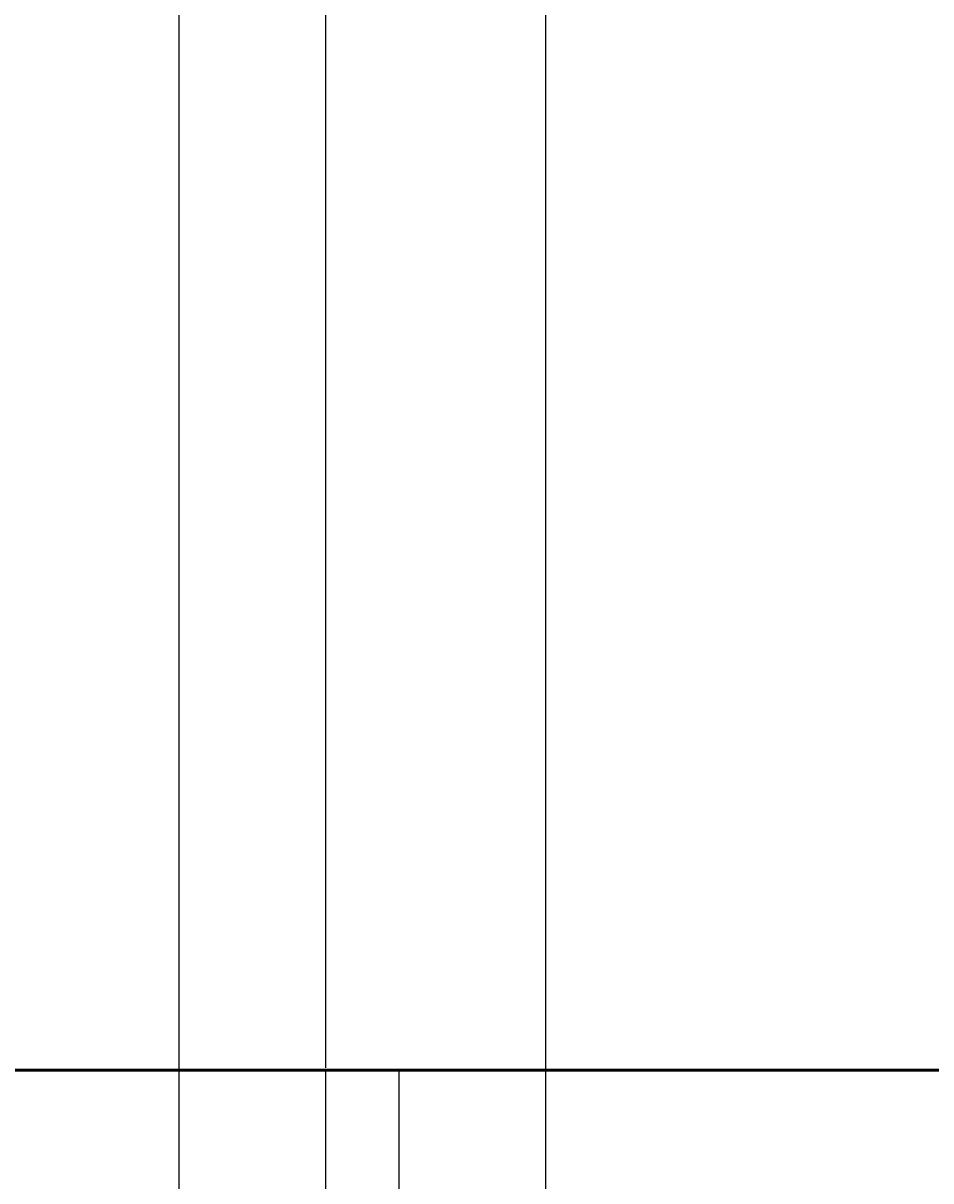
# Model space of a CAD drawing. Units: inches. Extents: x 37 to 824, y -700 to 234.
# Tile 29 of 77: x 202 to 227, y -269 to -237. Entities that reach past the tile are written whole.
import ezdxf

# ---------------------------------------------------------------- set-up
doc = ezdxf.new("R2010")
doc.units = ezdxf.units.IN
doc.header["$MEASUREMENT"] = 0
for name, color, linetype, lineweight in [('A-ANNO-DIMS', 2, 'Continuous', 18), ('A-GLAZ', 4, 'Continuous', 25), ('A-WALL', 2, 'Continuous', 50)]:
    doc.layers.add(name, color=color, linetype=linetype, lineweight=lineweight)
doc.styles.get("Standard").update_dxf_attribs({"font": 'arial.ttf'})
doc.dimstyles.get("Standard").update_dxf_attribs({"dimtxt": 0.18, "dimasz": 0.18, "dimexe": 0.18, "dimexo": 0.0625, "dimgap": 0.09, "dimtad": 0, "dimtih": 1, "dimtoh": 1, "dimdec": 1, "dimzin": 0, "dimdsep": 46, "dimlunit": 4, "dimtxsty": 'Standard', "dimcen": 0.09, "dimadec": 0, "dimazin": 0, "dimtfac": 1, "dimtdec": 1, "dimtofl": 0, "dimtmove": 0, "dimatfit": 3, "dimfxl": 1, "dimtolj": 1, "dimtzin": 0, "dimarcsym": 0})

# ---------------------------------------------------------------- blocks, each defined once
blk = doc.blocks.new('WIN-900')
for p, q in [((0, 9), (0, 0)), ((2, 9), (2, 0)), ((20, 9), (20, 0)), ((38, 9), (38, 0)), ((40, 9), (40, 0)), ((38, 5.5), (2, 5.5)), ((38, 3.5), (2, 3.5))]:
    blk.add_line(p, q)
blk = doc.blocks.new('*D80')
at = {"layer": 'A-ANNO-DIMS', "color": 0, "lineweight": -2, "ltscale": 0.5, "transparency": 16777216}
for p, q in [((170.077, -167.972), (170.077, -400.406)), ((250.19, -167.972), (250.19, -400.406)), ((170.257, -400.226), (209.804, -400.226)), ((250.01, -400.226), (210.463, -400.226))]:
    blk.add_line(p, q, dxfattribs=at)
at = {"layer": 'A-ANNO-DIMS', "color": 0, "ltscale": 0.5, "transparency": 16777216}
for points in [[(170.257, -400.196), (170.257, -400.256), (170.077, -400.226)], [(250.01, -400.196), (250.01, -400.256), (250.19, -400.226)]]:
    blk.add_solid(points, dxfattribs=at)
at = {"layer": 'Defpoints', "color": 0, "ltscale": 0.5, "transparency": 16777216}
for p in [(170.077, -167.91), (250.19, -167.91), (250.19, -400.226)]:
    blk.add_point(p, dxfattribs=at)
at = {"layer": 'A-ANNO-DIMS', "color": 0, "ltscale": 0.5, "transparency": 16777216, "insert": (210.133, -400.226), "char_height": 0.18, "attachment_point": 5}
blk.add_mtext('\\A1;6\'-8"', dxfattribs=at)
blk = doc.blocks.new('*D84')
at = {"layer": 'A-ANNO-DIMS', "color": 0, "lineweight": -2, "ltscale": 0.5, "transparency": 16777216}
for p, q in [((170.077, -265.847), (170.077, 234.17)), ((210.077, -265.847), (210.077, 234.17)), ((170.257, 233.99), (189.748, 233.99)), ((209.897, 233.99), (190.406, 233.99))]:
    blk.add_line(p, q, dxfattribs=at)
at = {"layer": 'A-ANNO-DIMS', "color": 0, "ltscale": 0.5, "transparency": 16777216}
for points in [[(170.257, 234.02), (170.257, 233.96), (170.077, 233.99)], [(209.897, 234.02), (209.897, 233.96), (210.077, 233.99)]]:
    blk.add_solid(points, dxfattribs=at)
at = {"layer": 'Defpoints', "color": 0, "ltscale": 0.5, "transparency": 16777216}
for p in [(210.077, 233.99), (170.077, -265.91), (210.077, -265.91)]:
    blk.add_point(p, dxfattribs=at)
at = {"layer": 'A-ANNO-DIMS', "color": 0, "ltscale": 0.5, "transparency": 16777216, "insert": (190.077, 233.99), "char_height": 0.18, "attachment_point": 5}
blk.add_mtext('\\A1;3\'-4"', dxfattribs=at)
blk = doc.blocks.new('*D85')
at = {"layer": 'A-ANNO-DIMS', "color": 0, "lineweight": -2, "ltscale": 0.5, "transparency": 16777216}
for p, q in [((170.077, -356.847), (170.077, 234.17)), ((206.077, -356.847), (206.077, 234.17)), ((170.257, 233.99), (187.748, 233.99)), ((205.897, 233.99), (188.406, 233.99))]:
    blk.add_line(p, q, dxfattribs=at)
at = {"layer": 'A-ANNO-DIMS', "color": 0, "ltscale": 0.5, "transparency": 16777216}
for points in [[(170.257, 234.02), (170.257, 233.96), (170.077, 233.99)], [(205.897, 234.02), (205.897, 233.96), (206.077, 233.99)]]:
    blk.add_solid(points, dxfattribs=at)
at = {"layer": 'Defpoints', "color": 0, "ltscale": 0.5, "transparency": 16777216}
for p in [(206.077, 233.99), (170.077, -356.91), (206.077, -356.91)]:
    blk.add_point(p, dxfattribs=at)
at = {"layer": 'A-ANNO-DIMS', "color": 0, "ltscale": 0.5, "transparency": 16777216, "insert": (188.077, 233.99), "char_height": 0.18, "attachment_point": 5}
blk.add_mtext('\\A1;3\'-0"', dxfattribs=at)
blk = doc.blocks.new('*D86')
at = {"layer": 'A-ANNO-DIMS', "color": 0, "lineweight": -2, "ltscale": 0.5, "transparency": 16777216}
for p, q in [((206.077, -356.847), (206.077, 234.17)), ((216.077, -356.847), (216.077, 234.17)), ((206.257, 233.99), (210.678, 233.99)), ((215.897, 233.99), (211.476, 233.99))]:
    blk.add_line(p, q, dxfattribs=at)
at = {"layer": 'A-ANNO-DIMS', "color": 0, "ltscale": 0.5, "transparency": 16777216}
for points in [[(206.257, 234.02), (206.257, 233.96), (206.077, 233.99)], [(215.897, 234.02), (215.897, 233.96), (216.077, 233.99)]]:
    blk.add_solid(points, dxfattribs=at)
at = {"layer": 'Defpoints', "color": 0, "ltscale": 0.5, "transparency": 16777216}
for p in [(216.077, 233.99), (206.077, -356.91), (216.077, -356.91)]:
    blk.add_point(p, dxfattribs=at)
at = {"layer": 'A-ANNO-DIMS', "color": 0, "ltscale": 0.5, "transparency": 16777216, "insert": (211.077, 233.99), "char_height": 0.18, "attachment_point": 5}
blk.add_mtext('\\A1;0\'-10"', dxfattribs=at)
blk = doc.blocks.new('*D87')
at = {"layer": 'A-ANNO-DIMS', "color": 0, "lineweight": -2, "ltscale": 0.5, "transparency": 16777216}
for p, q in [((216.077, -356.847), (216.077, 234.17)), ((296.077, -356.847), (296.077, 234.17)), ((216.257, 233.99), (255.747, 233.99)), ((295.897, 233.99), (256.407, 233.99))]:
    blk.add_line(p, q, dxfattribs=at)
at = {"layer": 'A-ANNO-DIMS', "color": 0, "ltscale": 0.5, "transparency": 16777216}
for points in [[(216.257, 234.02), (216.257, 233.96), (216.077, 233.99)], [(295.897, 234.02), (295.897, 233.96), (296.077, 233.99)]]:
    blk.add_solid(points, dxfattribs=at)
at = {"layer": 'Defpoints', "color": 0, "ltscale": 0.5, "transparency": 16777216}
for p in [(296.077, 233.99), (216.077, -356.91), (296.077, -356.91)]:
    blk.add_point(p, dxfattribs=at)
at = {"layer": 'A-ANNO-DIMS', "color": 0, "ltscale": 0.5, "transparency": 16777216, "insert": (256.077, 233.99), "char_height": 0.18, "attachment_point": 5}
blk.add_mtext('\\A1;6\'-8"', dxfattribs=at)

msp = doc.modelspace()

# ---------------------------------------------------------------- linework, layer by layer
at = {"layer": 'A-WALL'}
msp.add_line((290.077, -265.91), (170.077, -265.91), dxfattribs=at)

# ---------------------------------------------------------------- block references
at = {"layer": 'A-GLAZ', "rotation": 180}
msp.add_blockref('WIN-900', (250.077, -265.909), dxfattribs=at)

# ---------------------------------------------------------------- dimensions: what is measured, and where the dimension line sits
at = {"layer": 'A-ANNO-DIMS', "ltscale": 0.5}
for base, p1, p2, picture, middle in [((210.077, 233.99), (170.077, -265.91), (210.077, -265.91), '*D84', (190.077, 233.99)), ((206.077, 233.99), (170.077, -356.91), (206.077, -356.91), '*D85', (188.077, 233.99)), ((216.077, 233.99), (206.077, -356.91), (216.077, -356.91), '*D86', (211.077, 233.99)), ((296.077, 233.99), (216.077, -356.91), (296.077, -356.91), '*D87', (256.077, 233.99)), ((250.19, -400.226), (170.077, -167.91), (250.19, -167.91), '*D80', (210.133, -400.226))]:
    dim = msp.add_linear_dim(base=base, p1=p1, p2=p2, dimstyle='Standard', override={"dimdec": 1, "dimlfac": 1, "dimrnd": 0, "dimzin": 1, "dimdsep": 46, "dimlunit": 4, "dimfrac": 2}, dxfattribs=at)
    dim.commit()
    dim.dimension.update_dxf_attribs({"geometry": picture, "text_midpoint": middle})

doc.saveas('drawing.dxf')
